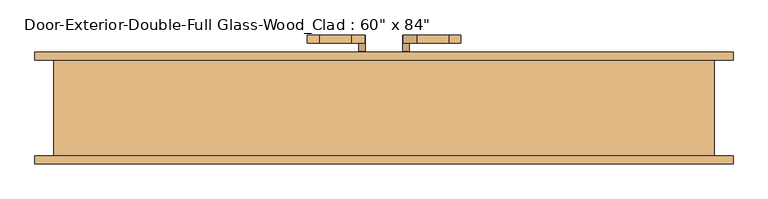
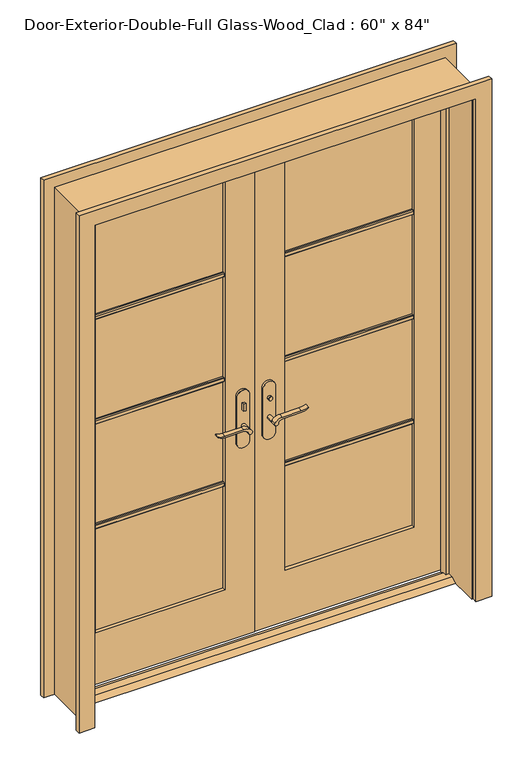
"""IFC4 building model written with IfcOpenShell, lengths in millimetres: door geometry."""

from ifc_helpers import new_model, si_unit, point, frame, frame_2d, origin, place, context, project, spatial, polyline, circle_curve, trimmed, segment, composite_curve, outline, extrude, faceted_brep, source, transform, mapped, element, save


def door_7ffae4ec(model_context):
    return source(origin(), model_context, "Body", "SolidModel", [
        extrude(outline(polyline([(19.05, 12.7), (53.975, 12.7), (79.375, 0.0), (-6.35, 0.0), (19.05, 12.7)])), frame((-762.0, 0.0, 0.0), z_axis=(1.0, 0.0, 0.0), x_axis=(0.0, 1.0, 0.0)), (0.0, 0.0, 1.0), 1524.0),
        extrude(outline(polyline([(-47.4019111, 56.2), (-57.4019111, 56.2), (-57.4019111, 66.2), (-47.4019111, 66.2), (-47.4019111, 56.2)])), frame((0.0, 0.0, 981.9), z_axis=(0.0, 0.0, 1.0), x_axis=(1.0, 0.0, 0.0)), (0.0, 0.0, 1.0), 30.0),
        extrude(outline(composite_curve([segment(trimmed(circle_curve(frame_2d((996.9, -52.4019111)), 8.0), [point((996.9, -60.4019111))], [point((996.9, -44.4019111))], False, "CARTESIAN"), True, "CONTINUOUS"), segment(trimmed(circle_curve(frame_2d((996.9, -52.4019111)), 8.0), [point((996.9, -44.4019111))], [point((996.9, -60.4019111))], False, "CARTESIAN"), True, "CONTINUOUS")], self_intersect=False)), frame((0.0, 121.125, 0.0), z_axis=(0.0, 1.0, 0.0), x_axis=(0.0, 0.0, 1.0)), (0.0, 0.0, 1.0), 10.0),
        extrude(outline(composite_curve([segment(trimmed(circle_curve(frame_2d((897.1555521, -76.0694241)), 37.2832219), [point((919.0523287, -45.8937749))], [point((934.4, -77.7693445))], False, "CARTESIAN"), True, "CONTINUOUS"), segment(polyline([(934.4, -77.7693445), (934.4, -154.045502)]), True, "CONTINUOUS"), segment(trimmed(circle_curve(frame_2d((1017.6850638, -153.9791202)), 83.2850902), [point((934.4, -154.045502))], [point((939.4, -182.4019111))], True, "CARTESIAN"), True, "CONTINUOUS"), segment(polyline([(939.4, -182.4019111), (936.6135558, -182.4019111)]), True, "CONTINUOUS"), segment(trimmed(circle_curve(frame_2d((986.6709207, -150.4622499)), 59.3791355), [point((936.6135558, -182.4019111))], [point((927.4, -154.045502))], False, "CARTESIAN"), True, "CONTINUOUS"), segment(polyline([(927.4, -154.045502), (927.4, -77.7881013)]), True, "CONTINUOUS"), segment(trimmed(circle_curve(frame_2d((909.2738613, -77.7881013)), 18.1261387), [point((927.4, -77.7881013))], [point((914.4, -60.4019111))], True, "CARTESIAN"), True, "CONTINUOUS"), segment(trimmed(circle_curve(frame_2d((914.4, -52.4019111)), 8.0), [point((914.4, -60.4019111))], [point((919.0523287, -45.8937749))], False, "CARTESIAN"), True, "CONTINUOUS")], self_intersect=False)), frame((0.0, 16.2, 0.0), z_axis=(0.0, 1.0, 0.0), x_axis=(0.0, 0.0, 1.0)), (0.0, 0.0, 1.0), 20.0),
        extrude(outline(composite_curve([segment(trimmed(circle_curve(frame_2d((914.4, -52.4019111)), 8.0), [point((914.3999903, -60.4019111))], [point((919.0523287, -45.8937749))], False, "CARTESIAN"), True, "CONTINUOUS"), segment(trimmed(circle_curve(frame_2d((897.1555521, -76.0694241)), 37.2832219), [point((919.0523287, -45.8937749))], [point((934.4, -77.7693445))], False, "CARTESIAN"), True, "CONTINUOUS"), segment(polyline([(934.4, -77.7693445), (934.4, -154.045502)]), True, "CONTINUOUS"), segment(trimmed(circle_curve(frame_2d((1017.6850638, -153.9791202)), 83.2850902), [point((934.4, -154.045502))], [point((939.4, -182.4019111))], True, "CARTESIAN"), True, "CONTINUOUS"), segment(polyline([(939.4, -182.4019111), (936.6135558, -182.4019111)]), True, "CONTINUOUS"), segment(trimmed(circle_curve(frame_2d((986.6709207, -150.4622499)), 59.3791355), [point((936.6135558, -182.4019111))], [point((927.4, -154.045502))], False, "CARTESIAN"), True, "CONTINUOUS"), segment(polyline([(927.4, -154.045502), (927.4, -77.788099)]), True, "CONTINUOUS"), segment(trimmed(circle_curve(frame_2d((909.2738682, -77.788099)), 18.1261318), [point((927.4, -77.788099))], [point((914.3999903, -60.4019111))], True, "CARTESIAN"), True, "CONTINUOUS")], self_intersect=False)), frame((0.0, 151.125, 0.0), z_axis=(0.0, 1.0, 0.0), x_axis=(0.0, 0.0, 1.0)), (0.0, 0.0, 1.0), 20.0),
        extrude(outline(composite_curve([segment(trimmed(circle_curve(frame_2d((914.4, -52.4019111)), 8.0), [point((914.4, -60.4019111))], [point((914.4, -44.4019111))], False, "CARTESIAN"), True, "CONTINUOUS"), segment(trimmed(circle_curve(frame_2d((914.4, -52.4019111)), 8.0), [point((914.4, -44.4019111))], [point((914.4, -60.4019111))], False, "CARTESIAN"), True, "CONTINUOUS")], self_intersect=False)), frame((0.0, 36.2, 0.0), z_axis=(0.0, 1.0, 0.0), x_axis=(0.0, 0.0, 1.0)), (0.0, 0.0, 1.0), 30.0),
        extrude(outline(composite_curve([segment(trimmed(circle_curve(frame_2d((914.4, -52.4019111)), 8.0), [point((914.4, -60.4019111))], [point((914.4, -44.4019111))], False, "CARTESIAN"), True, "CONTINUOUS"), segment(trimmed(circle_curve(frame_2d((914.4, -52.4019111)), 8.0), [point((914.4, -44.4019111))], [point((914.4, -60.4019111))], False, "CARTESIAN"), True, "CONTINUOUS")], self_intersect=False)), frame((0.0, 121.125, 0.0), z_axis=(0.0, 1.0, 0.0), x_axis=(0.0, 0.0, 1.0)), (0.0, 0.0, 1.0), 30.0),
        extrude(outline(composite_curve([segment(polyline([(844.4, -27.4019111), (1039.4, -27.4019111)]), True, "CONTINUOUS"), segment(trimmed(circle_curve(frame_2d((1039.4, -52.4019111)), 25.0), [point((1039.4, -27.4019111))], [point((1039.4, -77.4019111))], False, "CARTESIAN"), True, "CONTINUOUS"), segment(polyline([(1039.4, -77.4019111), (844.4, -77.4019111)]), True, "CONTINUOUS"), segment(trimmed(circle_curve(frame_2d((844.4, -52.4019111)), 25.0), [point((844.4, -77.4019111))], [point((844.4, -27.4019111))], False, "CARTESIAN"), True, "CONTINUOUS")], self_intersect=False)), frame((0.0, 66.2, 0.0), z_axis=(0.0, 1.0, 0.0), x_axis=(0.0, 0.0, 1.0)), (0.0, 0.0, 1.0), 10.0),
        extrude(outline(composite_curve([segment(polyline([(844.4, -27.4019111), (1039.4, -27.4019111)]), True, "CONTINUOUS"), segment(trimmed(circle_curve(frame_2d((1039.4, -52.4019111)), 25.0), [point((1039.4, -27.4019111))], [point((1039.4, -77.4019111))], False, "CARTESIAN"), True, "CONTINUOUS"), segment(polyline([(1039.4, -77.4019111), (844.4, -77.4019111)]), True, "CONTINUOUS"), segment(trimmed(circle_curve(frame_2d((844.4, -52.4019111)), 25.0), [point((844.4, -77.4019111))], [point((844.4, -27.4019111))], False, "CARTESIAN"), True, "CONTINUOUS")], self_intersect=False)), frame((0.0, 111.125, 0.0), z_axis=(0.0, 1.0, 0.0), x_axis=(0.0, 0.0, 1.0)), (0.0, 0.0, 1.0), 10.0),
        extrude(outline(polyline([(47.3875, 131.125), (57.3875, 131.125), (57.3875, 121.125), (47.3875, 121.125), (47.3875, 131.125)])), frame((0.0, 0.0, 981.9), z_axis=(0.0, 0.0, 1.0), x_axis=(1.0, 0.0, 0.0)), (0.0, 0.0, 1.0), 30.0),
        extrude(outline(composite_curve([segment(trimmed(circle_curve(frame_2d((996.9, 52.3875)), 8.0), [point((996.9, 60.3875))], [point((996.9, 44.3875))], False, "CARTESIAN"), True, "CONTINUOUS"), segment(trimmed(circle_curve(frame_2d((996.9, 52.3875)), 8.0), [point((996.9, 44.3875))], [point((996.9, 60.3875))], False, "CARTESIAN"), True, "CONTINUOUS")], self_intersect=False)), frame((0.0, 56.2, 0.0), z_axis=(0.0, 1.0, 0.0), x_axis=(0.0, 0.0, 1.0)), (0.0, 0.0, 1.0), 10.0),
        extrude(outline(composite_curve([segment(trimmed(circle_curve(frame_2d((914.4, 52.3875)), 8.0), [point((919.0523287, 45.8793637))], [point((914.4, 60.3875))], False, "CARTESIAN"), True, "CONTINUOUS"), segment(trimmed(circle_curve(frame_2d((909.2738613, 77.7736901)), 18.1261387), [point((914.4, 60.3875))], [point((927.4, 77.7736901))], True, "CARTESIAN"), True, "CONTINUOUS"), segment(polyline([(927.4, 77.7736901), (927.4, 154.0310909)]), True, "CONTINUOUS"), segment(trimmed(circle_curve(frame_2d((986.6709207, 150.4478388)), 59.3791355), [point((927.4, 154.0310909))], [point((936.6135558, 182.3875))], False, "CARTESIAN"), True, "CONTINUOUS"), segment(polyline([(936.6135558, 182.3875), (939.4, 182.3875)]), True, "CONTINUOUS"), segment(trimmed(circle_curve(frame_2d((1017.6850638, 153.9647091)), 83.2850902), [point((939.4, 182.3875))], [point((934.4, 154.0310909))], True, "CARTESIAN"), True, "CONTINUOUS"), segment(polyline([(934.4, 154.0310909), (934.4, 77.7549333)]), True, "CONTINUOUS"), segment(trimmed(circle_curve(frame_2d((897.1555521, 76.0550129)), 37.2832219), [point((934.4, 77.7549333))], [point((919.0523287, 45.8793637))], False, "CARTESIAN"), True, "CONTINUOUS")], self_intersect=False)), frame((0.0, 151.125, 0.0), z_axis=(0.0, 1.0, 0.0), x_axis=(0.0, 0.0, 1.0)), (0.0, 0.0, 1.0), 20.0),
        extrude(outline(composite_curve([segment(trimmed(circle_curve(frame_2d((909.2738682, 77.7736878)), 18.1261318), [point((914.3999903, 60.3875))], [point((927.4, 77.7736878))], True, "CARTESIAN"), True, "CONTINUOUS"), segment(polyline([(927.4, 77.7736878), (927.4, 154.0310909)]), True, "CONTINUOUS"), segment(trimmed(circle_curve(frame_2d((986.6709207, 150.4478388)), 59.3791355), [point((927.4, 154.0310909))], [point((936.6135558, 182.3875))], False, "CARTESIAN"), True, "CONTINUOUS"), segment(polyline([(936.6135558, 182.3875), (939.4, 182.3875)]), True, "CONTINUOUS"), segment(trimmed(circle_curve(frame_2d((1017.6850638, 153.9647091)), 83.2850902), [point((939.4, 182.3875))], [point((934.4, 154.0310909))], True, "CARTESIAN"), True, "CONTINUOUS"), segment(polyline([(934.4, 154.0310909), (934.4, 77.7549333)]), True, "CONTINUOUS"), segment(trimmed(circle_curve(frame_2d((897.1555521, 76.0550129)), 37.2832219), [point((934.4, 77.7549333))], [point((919.0523287, 45.8793637))], False, "CARTESIAN"), True, "CONTINUOUS"), segment(trimmed(circle_curve(frame_2d((914.4, 52.3875)), 8.0), [point((919.0523287, 45.8793637))], [point((914.3999903, 60.3875))], False, "CARTESIAN"), True, "CONTINUOUS")], self_intersect=False)), frame((0.0, 16.2, 0.0), z_axis=(0.0, 1.0, 0.0), x_axis=(0.0, 0.0, 1.0)), (0.0, 0.0, 1.0), 20.0),
        extrude(outline(composite_curve([segment(trimmed(circle_curve(frame_2d((914.4, 52.3875)), 8.0), [point((914.4, 60.3875))], [point((914.4, 44.3875))], False, "CARTESIAN"), True, "CONTINUOUS"), segment(trimmed(circle_curve(frame_2d((914.4, 52.3875)), 8.0), [point((914.4, 44.3875))], [point((914.4, 60.3875))], False, "CARTESIAN"), True, "CONTINUOUS")], self_intersect=False)), frame((0.0, 121.125, 0.0), z_axis=(0.0, 1.0, 0.0), x_axis=(0.0, 0.0, 1.0)), (0.0, 0.0, 1.0), 30.0),
        extrude(outline(composite_curve([segment(trimmed(circle_curve(frame_2d((914.4, 52.3875)), 8.0), [point((914.4, 60.3875))], [point((914.4, 44.3875))], False, "CARTESIAN"), True, "CONTINUOUS"), segment(trimmed(circle_curve(frame_2d((914.4, 52.3875)), 8.0), [point((914.4, 44.3875))], [point((914.4, 60.3875))], False, "CARTESIAN"), True, "CONTINUOUS")], self_intersect=False)), frame((0.0, 36.2, 0.0), z_axis=(0.0, 1.0, 0.0), x_axis=(0.0, 0.0, 1.0)), (0.0, 0.0, 1.0), 30.0),
        extrude(outline(composite_curve([segment(trimmed(circle_curve(frame_2d((844.4, 52.3875)), 25.0), [point((844.4, 27.3875))], [point((844.4, 77.3875))], False, "CARTESIAN"), True, "CONTINUOUS"), segment(polyline([(844.4, 77.3875), (1039.4, 77.3875)]), True, "CONTINUOUS"), segment(trimmed(circle_curve(frame_2d((1039.4, 52.3875)), 25.0), [point((1039.4, 77.3875))], [point((1039.4, 27.3875))], False, "CARTESIAN"), True, "CONTINUOUS"), segment(polyline([(1039.4, 27.3875), (844.4, 27.3875)]), True, "CONTINUOUS")], self_intersect=False)), frame((0.0, 111.125, 0.0), z_axis=(0.0, 1.0, 0.0), x_axis=(0.0, 0.0, 1.0)), (0.0, 0.0, 1.0), 10.0),
        extrude(outline(composite_curve([segment(trimmed(circle_curve(frame_2d((844.4, 52.3875)), 25.0), [point((844.4, 27.3875))], [point((844.4, 77.3875))], False, "CARTESIAN"), True, "CONTINUOUS"), segment(polyline([(844.4, 77.3875), (1039.4, 77.3875)]), True, "CONTINUOUS"), segment(trimmed(circle_curve(frame_2d((1039.4, 52.3875)), 25.0), [point((1039.4, 77.3875))], [point((1039.4, 27.3875))], False, "CARTESIAN"), True, "CONTINUOUS"), segment(polyline([(1039.4, 27.3875), (844.4, 27.3875)]), True, "CONTINUOUS")], self_intersect=False)), frame((0.0, 66.2, 0.0), z_axis=(0.0, 1.0, 0.0), x_axis=(0.0, 0.0, 1.0)), (0.0, 0.0, 1.0), 10.0),
        extrude(outline(polyline([(90.17, 1578.371875), (90.17, 1559.321875), (83.82, 1559.321875), (80.645, 1562.496875), (80.645, 1575.196875), (83.82, 1578.371875), (90.17, 1578.371875)])), frame((120.65, 0.0, 0.0), z_axis=(1.0, 0.0, 0.0), x_axis=(0.0, 1.0, 0.0)), (0.0, 0.0, 1.0), 520.7),
        extrude(outline(polyline([(90.17, 1132.68125), (90.17, 1113.63125), (83.82, 1113.63125), (80.645, 1116.80625), (80.645, 1129.50625), (83.82, 1132.68125), (90.17, 1132.68125)])), frame((120.65, 0.0, 0.0), z_axis=(1.0, 0.0, 0.0), x_axis=(0.0, 1.0, 0.0)), (0.0, 0.0, 1.0), 520.7),
        extrude(outline(polyline([(90.17, 686.990625), (90.17, 667.940625), (83.82, 667.940625), (80.645, 671.115625), (80.645, 683.815625), (83.82, 686.990625), (90.17, 686.990625)])), frame((120.65, 0.0, 0.0), z_axis=(1.0, 0.0, 0.0), x_axis=(0.0, 1.0, 0.0)), (0.0, 0.0, 1.0), 520.7),
        extrude(outline(polyline([(97.155, 1578.371875), (103.505, 1578.371875), (106.68, 1575.196875), (106.68, 1562.496875), (103.505, 1559.321875), (97.155, 1559.321875), (97.155, 1578.371875)])), frame((-641.35, 0.0, 0.0), z_axis=(1.0, 0.0, 0.0), x_axis=(0.0, 1.0, 0.0)), (0.0, 0.0, 1.0), 520.7),
        extrude(outline(polyline([(97.155, 1132.68125), (103.505, 1132.68125), (106.68, 1129.50625), (106.68, 1116.80625), (103.505, 1113.63125), (97.155, 1113.63125), (97.155, 1132.68125)])), frame((-641.35, 0.0, 0.0), z_axis=(1.0, 0.0, 0.0), x_axis=(0.0, 1.0, 0.0)), (0.0, 0.0, 1.0), 520.7),
        extrude(outline(polyline([(97.155, 686.990625), (103.505, 686.990625), (106.68, 683.815625), (106.68, 671.115625), (103.505, 667.940625), (97.155, 667.940625), (97.155, 686.990625)])), frame((-641.35, 0.0, 0.0), z_axis=(1.0, 0.0, 0.0), x_axis=(0.0, 1.0, 0.0)), (0.0, 0.0, 1.0), 520.7),
        extrude(outline(polyline([(97.155, 1578.371875), (103.505, 1578.371875), (106.68, 1575.196875), (106.68, 1562.496875), (103.505, 1559.321875), (97.155, 1559.321875), (97.155, 1578.371875)])), frame((120.65, 0.0, 0.0), z_axis=(1.0, 0.0, 0.0), x_axis=(0.0, 1.0, 0.0)), (0.0, 0.0, 1.0), 520.7),
        extrude(outline(polyline([(97.155, 1132.68125), (103.505, 1132.68125), (106.68, 1129.50625), (106.68, 1116.80625), (103.505, 1113.63125), (97.155, 1113.63125), (97.155, 1132.68125)])), frame((120.65, 0.0, 0.0), z_axis=(1.0, 0.0, 0.0), x_axis=(0.0, 1.0, 0.0)), (0.0, 0.0, 1.0), 520.7),
        extrude(outline(polyline([(97.155, 686.990625), (103.505, 686.990625), (106.68, 683.815625), (106.68, 671.115625), (103.505, 667.940625), (97.155, 667.940625), (97.155, 686.990625)])), frame((120.65, 0.0, 0.0), z_axis=(1.0, 0.0, 0.0), x_axis=(0.0, 1.0, 0.0)), (0.0, 0.0, 1.0), 520.7),
        extrude(outline(polyline([(90.17, 1578.371875), (90.17, 1559.321875), (83.82, 1559.321875), (80.645, 1562.496875), (80.645, 1575.196875), (83.82, 1578.371875), (90.17, 1578.371875)])), frame((-641.35, 0.0, 0.0), z_axis=(1.0, 0.0, 0.0), x_axis=(0.0, 1.0, 0.0)), (0.0, 0.0, 1.0), 520.7),
        extrude(outline(polyline([(90.17, 1132.68125), (90.17, 1113.63125), (83.82, 1113.63125), (80.645, 1116.80625), (80.645, 1129.50625), (83.82, 1132.68125), (90.17, 1132.68125)])), frame((-641.35, 0.0, 0.0), z_axis=(1.0, 0.0, 0.0), x_axis=(0.0, 1.0, 0.0)), (0.0, 0.0, 1.0), 520.7),
        extrude(outline(polyline([(90.17, 686.990625), (90.17, 667.940625), (83.82, 667.940625), (80.645, 671.115625), (80.645, 683.815625), (83.82, 686.990625), (90.17, 686.990625)])), frame((-641.35, 0.0, 0.0), z_axis=(1.0, 0.0, 0.0), x_axis=(0.0, 1.0, 0.0)), (0.0, 0.0, 1.0), 520.7),
        extrude(outline(polyline([(0.0, 768.35), (0.0, 831.85), (2203.45, 831.85), (2203.45, -831.85), (0.0, -831.85), (0.0, -768.35), (2139.95, -768.35), (2139.95, 768.35), (0.0, 768.35)])), frame((0.0, -136.525, 0.0), z_axis=(0.0, 1.0, 0.0), x_axis=(0.0, 0.0, 1.0)), (0.0, 0.0, 1.0), 19.05),
        extrude(outline(polyline([(0.0, 768.35), (0.0, 831.85), (2203.45, 831.85), (2203.45, -831.85), (0.0, -831.85), (0.0, -768.35), (2139.95, -768.35), (2139.95, 768.35), (0.0, 768.35)])), frame((0.0, 111.125, 0.0), z_axis=(0.0, 1.0, 0.0), x_axis=(0.0, 0.0, 1.0)), (0.0, 0.0, 1.0), 19.05),
        faceted_brep([(787.4, 111.125, 0.0), (787.4, -117.475, 0.0), (762.0, -117.475, 0.0), (762.0, 41.275, 0.0), (749.3, 41.275, 0.0), (749.3, 76.2, 0.0), (762.0, 76.2, 0.0), (762.0, 111.125, 0.0), (787.4, 111.125, 2159.0), (787.4, -117.475, 2159.0), (-787.4, -117.475, 2159.0), (-787.4, -117.475, 0.0), (-762.0, -117.475, 0.0), (-762.0, -117.475, 2133.6), (762.0, -117.475, 2133.6), (762.0, 41.275, 2133.6), (-762.0, 41.275, 2133.6), (-762.0, 41.275, 0.0), (-749.3, 41.275, 0.0), (-749.3, 41.275, 2120.9), (749.3, 41.275, 2120.9), (749.3, 76.2, 2120.9), (1.5875, 76.2, 2120.9), (-1.6019111, 76.2, 2120.9), (-749.3, 76.2, 2120.9), (-749.3, 76.2, 0.0), (-762.0, 76.2, 0.0), (-762.0, 76.2, 2133.6), (-1.6019111, 76.2, 2133.6), (1.5875, 76.2, 2133.6), (762.0, 76.2, 2133.6), (762.0, 111.125, 2133.6), (1.5875, 111.125, 2133.6), (-1.6019111, 111.125, 2133.6), (-762.0, 111.125, 2133.6), (-762.0, 111.125, 0.0), (-787.4, 111.125, 0.0), (-787.4, 111.125, 2159.0)], [[[0, 1, 2, 3, 4, 5, 6, 7]], [[1, 0, 8, 9]], [[2, 1, 9, 10, 11, 12, 13, 14]], [[3, 2, 14, 15]], [[4, 3, 15, 16, 17, 18, 19, 20]], [[5, 4, 20, 21]], [[6, 5, 21, 22, 23, 24, 25, 26, 27, 28, 29, 30]], [[7, 6, 30, 31]], [[0, 7, 31, 32, 33, 34, 35, 36, 37, 8]], [[9, 8, 37, 10]], [[14, 13, 16, 15]], [[20, 19, 24, 23, 22, 21]], [[31, 30, 29, 28, 27, 34, 33, 32]], [[12, 11, 36, 35, 26, 25, 18, 17]], [[11, 10, 37, 36]], [[13, 12, 17, 16]], [[19, 18, 25, 24]], [[27, 26, 35, 34]]]),
        extrude(outline(polyline([(12.7, 762.0), (2133.6, 762.0), (2133.6, 1.5875), (12.7, 1.5875), (12.7, 762.0)]), holes=[polyline([(2014.5375, 120.65), (2014.5375, 641.35), (231.775, 641.35), (231.775, 120.65), (2014.5375, 120.65)])]), frame((0.0, 76.2, 0.0), z_axis=(0.0, 1.0, 0.0), x_axis=(0.0, 0.0, 1.0)), (0.0, 0.0, 1.0), 34.925),
        extrude(outline(polyline([(2133.6, -762.0), (12.7, -762.0), (12.7, -1.6019111), (2133.6, -1.6019111), (2133.6, -762.0)]), holes=[polyline([(231.775, -641.35), (2014.5375, -641.35), (2014.5375, -120.65), (231.775, -120.65), (231.775, -641.35)])]), frame((0.0, 76.2, 0.0), z_axis=(0.0, 1.0, 0.0), x_axis=(0.0, 0.0, 1.0)), (0.0, 0.0, 1.0), 34.925),
        extrude(outline(polyline([(641.35, 90.17), (120.65, 90.17), (120.65, 97.155), (641.35, 97.155), (641.35, 90.17)])), frame((0.0, 0.0, 231.775), z_axis=(0.0, 0.0, 1.0), x_axis=(1.0, 0.0, 0.0)), (0.0, 0.0, 1.0), 1782.7625),
        extrude(outline(polyline([(-120.65, 90.17), (-641.35, 90.17), (-641.35, 97.155), (-120.65, 97.155), (-120.65, 90.17)])), frame((0.0, 0.0, 231.775), z_axis=(0.0, 0.0, 1.0), x_axis=(1.0, 0.0, 0.0)), (0.0, 0.0, 1.0), 1782.7625),
    ])


if __name__ == "__main__":
    model = new_model("IFC4")
    model_context = context("Model", 3, world=origin())
    ifc_project = project(units=[si_unit("LENGTHUNIT", "METRE", prefix="MILLI")], contexts=[model_context])
    site = spatial("IfcSite", under=ifc_project)
    building = spatial("IfcBuilding", under=site)
    placement = place(None, origin())
    door_shape = door_7ffae4ec(model_context)
    element("IfcDoor", 1, ObjectType="Door-Exterior-Double-Full Glass-Wood_Clad : 60\" x 84\"", at=placement, inside=building, context=model_context, shape_type="MappedRepresentation", body=[
        mapped(door_shape, transform((0.0, 0.0, 0.0), x_axis=(1.0, 0.0, 0.0), y_axis=(0.0, 1.0, 0.0), z_axis=(0.0, 0.0, 1.0))),
    ])
    save(model, "model.ifc")

# Revit data of these elements
# Type "Door-Exterior-Double-Full Glass-Wood_Clad : 60\" x 84\""
#   Type Mark = "9"
#   Assembly Code = "B2030100"
#   Analytic Construction = "French door, wood frame with double glass"
#   Top Rail = 0' - 4 11/16"
#   Threshold Offset [instance default] = 0' - 0 1/2"
#   Thickness = 0' - 1 3/8"
#   Thermal Resistance (R) = 1.9158 (h·ft²·°F)/BTU
#   Swing Angle [instance default] = 90.00°
#   Stiles = 0' - 4 3/4"
#   Rough Width = 5' - 2"
#   Rough Height = 7' - 1"
#   Panel Width = 2' - 6"
#   Door Offset [instance default] = 0' - 0"
#   Height = 7' - 0"
#   Width = 5' - 0"
#   Heat Transfer Coefficient (U) = 0.5220 BTU/(h·ft²·°F)
#   Bottom Rail = 0' - 9 1/8"
#   Exterior Trim [instance default] = yes
#   Threshold [instance default] = yes
#   Show Grill [instance default] = yes
#   Function = 1
#   Trim Material = Cherry
#   Threshold Material = Cherry
#   Panel Material = Cherry
#   Glazing = Glass
#   Frame Material = Cherry
#   Door Handle Material = Aluminum
#   Visual Light Transmittance = 0
#   Solar Heat Gain Coefficient = 0
#   Wall Closure = (empty or 0)
#   Construction Type = (empty or 0)
# Element 1 (IfcDoor, "Door-Exterior-Double-Full Glass-Wood_Clad : 60\" x 84\"")
#   Materials on its faces: "Cherry", "Aluminum", "Glass"
# Materials
#   "Cherry": class "Wood", colour RGB 226 177 128, transparency 0, Description = "Prunus Serotina", Cost = 0
#   "Glass": class "Glass", colour RGB 0 128 192, transparency 0.75, Description = "Soda Lime Glass", Cost = 0
#   "Aluminum": class "Metal", colour RGB 247 247 247, transparency 0, Description = "Aluminum 6061", Cost = 0
